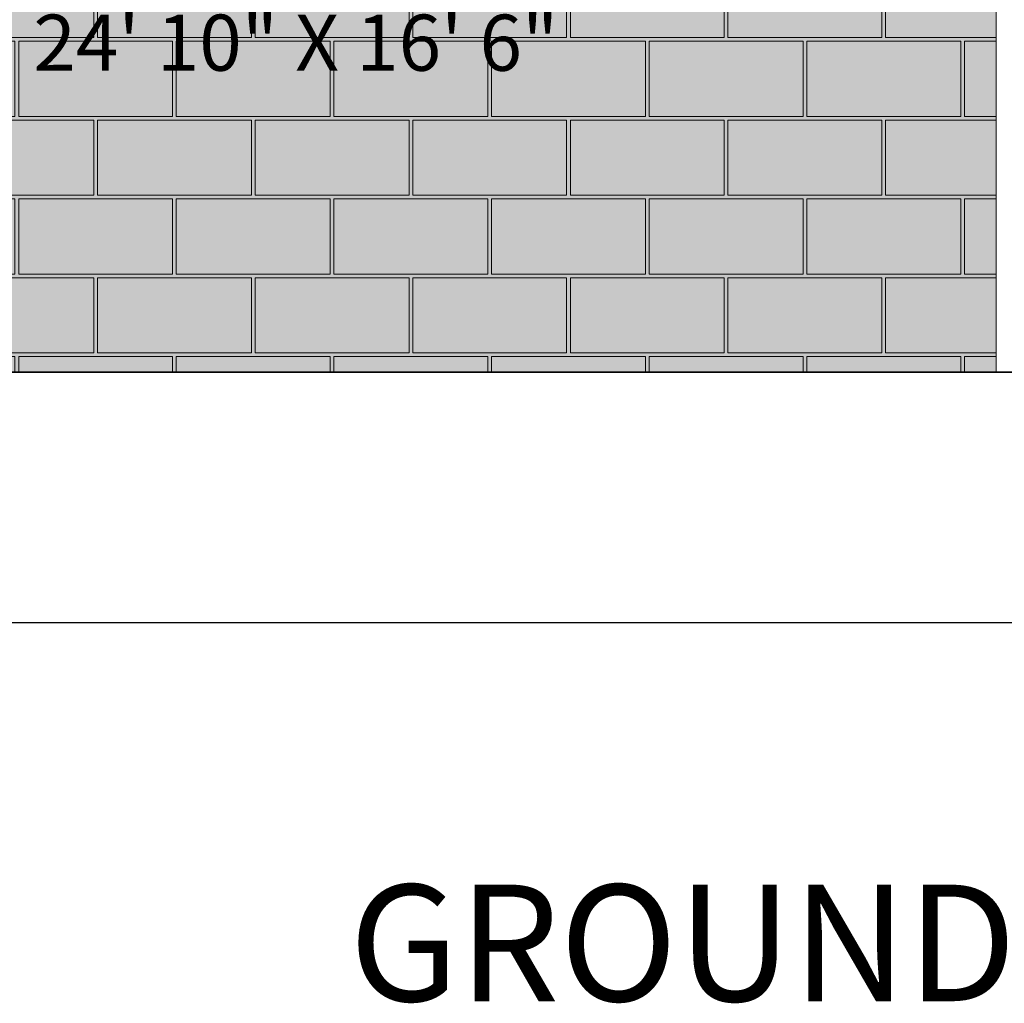
# Model space of a CAD drawing. Units: inches. Extents: x 1704 to 6393, y -157 to 1172.
# Tile 8 of 122: x 2035 to 2275, y -157 to 82. Entities that reach past the tile are written whole.
import ezdxf

# ---------------------------------------------------------------- set-up
doc = ezdxf.new("R2010")
doc.units = ezdxf.units.IN
doc.header["$MEASUREMENT"] = 0
for name, color, linetype, lineweight in [('A-ANNO-DIMS', 7, 'Continuous', 13), ('A-ANNO-TEXT', 7, 'Continuous', 25), ('C-PROP', 7, 'Continuous', 35), ('L-HRDS', 8, 'Continuous', 18), ('L-PVMT-PATT', 8, 'Continuous', 13)]:
    doc.layers.add(name, color=color, linetype=linetype, lineweight=lineweight)
doc.layers.add('L-HRDS-PATT', color=9, linetype='Continuous', lineweight=13, true_color=0xc5c1ba)
doc.styles.get("Standard").update_dxf_attribs({"font": 'arial.ttf'})
doc.dimstyles.get("Standard").update_dxf_attribs({"dimtxt": 6, "dimasz": 2, "dimexe": 0.18, "dimexo": 0.0625, "dimgap": 0.09, "dimtad": 0, "dimtih": 1, "dimtoh": 1, "dimdec": 1, "dimzin": 0, "dimdsep": 46, "dimlunit": 3, "dimtxsty": 'Standard', "dimblk": 'ARCHTICK', "dimcen": 0.09, "dimadec": 0, "dimazin": 0, "dimtfac": 1, "dimtdec": 1, "dimtofl": 0, "dimtmove": 0, "dimatfit": 3, "dimfxl": 1, "dimtolj": 1, "dimtzin": 0, "dimarcsym": 0})

# ---------------------------------------------------------------- blocks, each defined once
blk = doc.blocks.new('_ArchTick')
at = {"color": 0, "linetype": 'ByBlock', "const_width": 0.15}
blk.add_lwpolyline([(-0.5, -0.5), (0.5, 0.5)], dxfattribs=at)
blk = doc.blocks.new('*D90')
at = {"layer": 'A-ANNO-DIMS', "color": 0, "lineweight": -2, "transparency": 16777216}
for p, q in [((1898.35, -3.85), (1898.35, -64.97)), ((2723.35, -3.85), (2723.35, -64.97)), ((1898.35, -64.79), (2304.1, -64.79)), ((2723.35, -64.79), (2317.59, -64.79))]:
    blk.add_line(p, q, dxfattribs=at)
at = {"layer": 'Defpoints', "color": 0, "lineweight": -3, "transparency": 16777216}
for p in [(1898.35, -3.79), (2723.35, -3.79), (2723.35, -64.79)]:
    blk.add_point(p, dxfattribs=at)
at = {"layer": 'A-ANNO-DIMS', "color": 0, "lineweight": -2, "transparency": 16777216, "xscale": 2, "yscale": 2, "zscale": 2, "rotation": 180}
blk.add_blockref('_ArchTick', (1898.35, -64.79), dxfattribs=at)
at = {"layer": 'A-ANNO-DIMS', "color": 0, "lineweight": -2, "transparency": 16777216, "xscale": 2, "yscale": 2, "zscale": 2}
blk.add_blockref('_ArchTick', (2723.35, -64.79), dxfattribs=at)
at = {"layer": 'A-ANNO-DIMS', "color": 0, "transparency": 16777216, "insert": (2310.85, -64.79), "char_height": 6, "attachment_point": 5}
blk.add_mtext('\\A1;825', dxfattribs=at)

msp = doc.modelspace()

# ---------------------------------------------------------------- hatches: boundary and pattern name
at = {"layer": 'L-HRDS-PATT', "transparency": 33554646}
h = msp.add_hatch(color=256, dxfattribs=at)
h.dxf.hatch_style = 1
h.paths.add_polyline_path([(2273.349, 194.213), (2269.516, 194.213), (2268.215, 194.213), (2230.482, 194.213), (2229.181, 194.213), (2225.349, 194.213), (2049.349, 194.213), (2049.349, 202.213), (1975.349, 202.213), (1975.349, -3.787), (2273.349, -3.787)])
at = {"layer": 'L-PVMT-PATT', "transparency": 33554643}
h = msp.add_hatch(dxfattribs=at)
h.set_pattern_fill('AR-B816C', color=256, scale=2.4)
h.paths.add_polyline_path([(2273.349, 194.213), (2269.516, 194.213), (2268.215, 194.213), (2230.482, 194.213), (2229.181, 194.213), (2225.349, 194.213), (2049.349, 194.213), (2049.349, 202.213), (1975.349, 202.213), (1975.349, -3.787), (2273.349, -3.787)])

# ---------------------------------------------------------------- linework, layer by layer
at = {"layer": 'C-PROP'}
msp.add_line((2723.349, -3.787), (1898.349, -3.787), dxfattribs=at)
at = {"layer": 'L-HRDS'}
msp.add_line((2273.349, 194.213), (2273.349, -3.787), dxfattribs=at)

# ---------------------------------------------------------------- texts
at = {"layer": 'A-ANNO-DIMS'}
msp.add_text('24\' 10" X 16\' 6"', height=13.6672, dxfattribs=at).set_placement((2038.807, 69.622))
at = {"layer": 'A-ANNO-TEXT'}
msp.add_text('GROUND FLOOR', height=28.38733, dxfattribs=at).set_placement((2115.73, -156.99))

# ---------------------------------------------------------------- dimensions: what is measured, and where the dimension line sits
at = {"layer": 'A-ANNO-DIMS'}
dim = msp.add_linear_dim(base=(2723.349, -64.787), p1=(1898.349, -3.787), p2=(2723.349, -3.787), dimstyle='Standard', override={"dimdec": 0, "dimlfac": 1, "dimrnd": 0, "dimzin": 0, "dimdsep": 46, "dimlunit": 2}, dxfattribs=at)
dim.commit()
dim.dimension.update_dxf_attribs({"geometry": '*D90', "text_midpoint": (2310.849, -64.787)})

doc.saveas('drawing.dxf')
